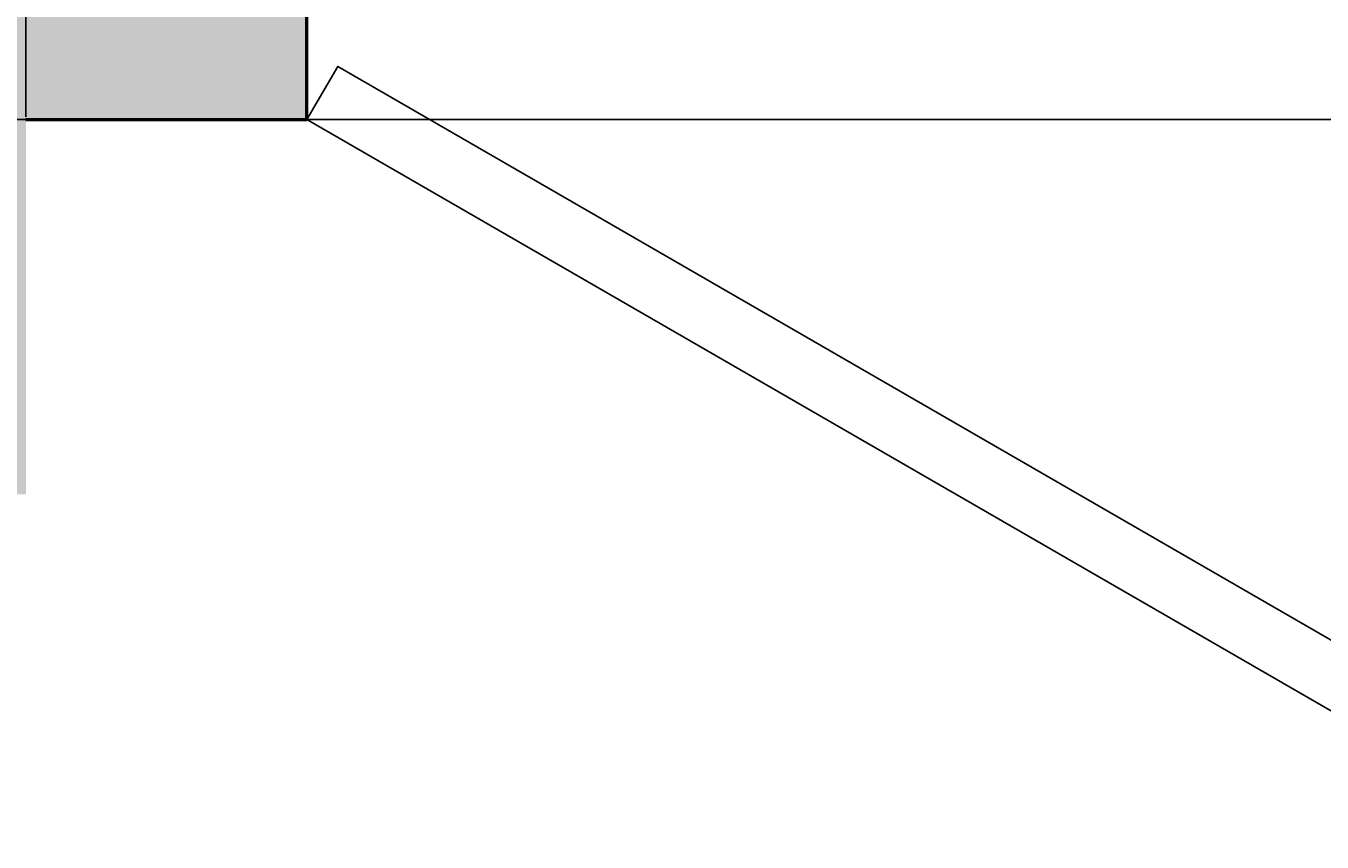
# Model space of a CAD drawing. Units: inches. Extents: x 2231 to 2461, y 2045 to 2455.
# Tile 12 of 95: x 2299 to 2326, y 2167 to 2185. Entities that reach past the tile are written whole.
import ezdxf

# ---------------------------------------------------------------- set-up
doc = ezdxf.new("R2010")
doc.units = ezdxf.units.IN
for name, color, linetype, lineweight in [('A-ANNO-DIMS', 2, 'Continuous', 18), ('A-DOOR', 3, 'Continuous', 25), ('A-WALL', 7, 'Continuous', 50)]:
    doc.layers.add(name, color=color, linetype=linetype, lineweight=lineweight)
doc.layers.add('A-WALL-PATT', color=18, linetype='Continuous', lineweight=13, true_color=0x000000)
doc.styles.get("Standard").update_dxf_attribs({"font": 'arial.ttf'})
doc.dimstyles.get("Standard").update_dxf_attribs({"dimtxt": 0.18, "dimasz": 0.18, "dimexe": 0.18, "dimexo": 0.0625, "dimgap": 0.09, "dimtad": 0, "dimtih": 1, "dimtoh": 1, "dimdec": 4, "dimzin": 0, "dimdsep": 46, "dimtxsty": 'Standard', "dimcen": 0.09, "dimadec": 0, "dimazin": 0, "dimtfac": 1, "dimtdec": 4, "dimtofl": 0, "dimtmove": 0, "dimatfit": 3, "dimfxl": 1, "dimtolj": 1, "dimtzin": 0, "dimarcsym": 0})

# ---------------------------------------------------------------- blocks, each defined once
blk = doc.blocks.new('*U4')
blk.add_line((0, 0), (0, 6))
blk.add_lwpolyline([(0, 0), (34.641, -20), (35.516, -18.484), (0.875, 1.516)], close=True)
blk = doc.blocks.new('*D49')
at = {"layer": 'A-ANNO-DIMS', "color": 0, "lineweight": -2, "transparency": 16777216}
for p, q in [((2298.794, 2182.895), (2298.794, 2454.645)), ((2304.794, 2182.895), (2304.794, 2454.645)), ((2298.974, 2454.465), (2301.644, 2454.465)), ((2304.614, 2454.465), (2301.943, 2454.465))]:
    blk.add_line(p, q, dxfattribs=at)
at = {"layer": 'A-ANNO-DIMS', "color": 0, "transparency": 16777216}
for points in [[(2298.974, 2454.495), (2298.974, 2454.435), (2298.794, 2454.465)], [(2304.614, 2454.495), (2304.614, 2454.435), (2304.794, 2454.465)]]:
    blk.add_solid(points, dxfattribs=at)
at = {"layer": 'Defpoints', "color": 0, "transparency": 16777216}
for p in [(2304.794, 2454.465), (2298.794, 2182.833), (2304.794, 2182.833)]:
    blk.add_point(p, dxfattribs=at)
at = {"layer": 'A-ANNO-DIMS', "color": 0, "transparency": 16777216, "insert": (2301.794, 2454.465), "char_height": 0.18, "attachment_point": 5}
blk.add_mtext('\\A1;6', dxfattribs=at)
blk = doc.blocks.new('*D50')
at = {"layer": 'A-ANNO-DIMS', "color": 0, "lineweight": -2, "transparency": 16777216}
for p, q in [((2304.794, 2182.895), (2304.794, 2454.645)), ((2334.794, 2182.895), (2334.794, 2454.645)), ((2304.974, 2454.465), (2319.575, 2454.465)), ((2334.614, 2454.465), (2320.012, 2454.465))]:
    blk.add_line(p, q, dxfattribs=at)
at = {"layer": 'A-ANNO-DIMS', "color": 0, "transparency": 16777216}
for points in [[(2304.974, 2454.495), (2304.974, 2454.435), (2304.794, 2454.465)], [(2334.614, 2454.495), (2334.614, 2454.435), (2334.794, 2454.465)]]:
    blk.add_solid(points, dxfattribs=at)
at = {"layer": 'Defpoints', "color": 0, "transparency": 16777216}
for p in [(2334.794, 2454.465), (2304.794, 2182.833), (2334.794, 2182.833)]:
    blk.add_point(p, dxfattribs=at)
at = {"layer": 'A-ANNO-DIMS', "color": 0, "transparency": 16777216, "insert": (2319.794, 2454.465), "char_height": 0.18, "attachment_point": 5}
blk.add_mtext('\\A1;30', dxfattribs=at)
blk = doc.blocks.new('*D51')
at = {"layer": 'A-ANNO-DIMS', "color": 0, "lineweight": -2, "transparency": 16777216}
for p, q in [((2258.794, 2306.77), (2258.794, 2044.803)), ((2330.794, 2306.77), (2330.794, 2044.803)), ((2258.974, 2044.983), (2294.576, 2044.983)), ((2330.614, 2044.983), (2295.011, 2044.983))]:
    blk.add_line(p, q, dxfattribs=at)
at = {"layer": 'A-ANNO-DIMS', "color": 0, "transparency": 16777216}
for points in [[(2258.974, 2045.013), (2258.974, 2044.953), (2258.794, 2044.983)], [(2330.614, 2045.013), (2330.614, 2044.953), (2330.794, 2044.983)]]:
    blk.add_solid(points, dxfattribs=at)
at = {"layer": 'Defpoints', "color": 0, "transparency": 16777216}
for p in [(2258.794, 2306.833), (2330.794, 2306.833), (2330.794, 2044.983)]:
    blk.add_point(p, dxfattribs=at)
at = {"layer": 'A-ANNO-DIMS', "color": 0, "transparency": 16777216, "insert": (2294.794, 2044.983), "char_height": 0.18, "attachment_point": 5}
blk.add_mtext('\\A1;72', dxfattribs=at)
blk = doc.blocks.new('*D60')
at = {"layer": 'A-ANNO-DIMS', "color": 0, "lineweight": -2, "transparency": 16777216}
for p, q in [((2432.731, 2182.833), (2230.981, 2182.833)), ((2231.161, 2182.653), (2231.161, 2166.906)), ((2231.161, 2150.795), (2231.161, 2166.542)), ((2432.731, 2150.615), (2230.981, 2150.615))]:
    blk.add_line(p, q, dxfattribs=at)
at = {"layer": 'A-ANNO-DIMS', "color": 0, "transparency": 16777216}
for points in [[(2231.131, 2182.653), (2231.191, 2182.653), (2231.161, 2182.833)], [(2231.131, 2150.795), (2231.191, 2150.795), (2231.161, 2150.615)]]:
    blk.add_solid(points, dxfattribs=at)
at = {"layer": 'Defpoints', "color": 0, "transparency": 16777216}
for p in [(2231.161, 2182.833), (2432.794, 2182.833), (2432.794, 2150.615)]:
    blk.add_point(p, dxfattribs=at)
at = {"layer": 'A-ANNO-DIMS', "color": 0, "transparency": 16777216, "insert": (2231.161, 2166.724), "char_height": 0.18, "attachment_point": 5}
blk.add_mtext('\\A1;32.22', dxfattribs=at)
blk = doc.blocks.new('*D65')
at = {"layer": 'A-ANNO-DIMS', "color": 0, "lineweight": -2, "transparency": 16777216}
for p, q in [((2285.635, 2189.285), (2285.635, 2044.803)), ((2340.667, 2189.285), (2340.667, 2044.803)), ((2285.815, 2044.983), (2312.758, 2044.983)), ((2340.487, 2044.983), (2313.545, 2044.983))]:
    blk.add_line(p, q, dxfattribs=at)
at = {"layer": 'A-ANNO-DIMS', "color": 0, "transparency": 16777216}
for points in [[(2285.815, 2045.013), (2285.815, 2044.953), (2285.635, 2044.983)], [(2340.487, 2045.013), (2340.487, 2044.953), (2340.667, 2044.983)]]:
    blk.add_solid(points, dxfattribs=at)
at = {"layer": 'Defpoints', "color": 0, "transparency": 16777216}
for p in [(2285.635, 2189.348), (2340.667, 2189.348), (2340.667, 2044.983)]:
    blk.add_point(p, dxfattribs=at)
at = {"layer": 'A-ANNO-DIMS', "color": 0, "transparency": 16777216, "insert": (2313.151, 2044.983), "char_height": 0.18, "attachment_point": 5}
blk.add_mtext('\\A1;55.03', dxfattribs=at)

msp = doc.modelspace()

# ---------------------------------------------------------------- hatches: boundary and pattern name
at = {"layer": 'A-WALL-PATT'}
h = msp.add_hatch(color=256, dxfattribs=at)
h.dxf.hatch_style = 1
h.paths.add_polyline_path([(2441.7935, 2269.1535), (2432.7935, 2269.1535), (2432.7935, 2186.8328), (2396.7935, 2186.8328), (2396.7935, 2286.8328), (2394.7935, 2286.8328), (2394.7935, 2186.8328), (2334.7935, 2186.8328), (2334.7935, 2182.8328), (2432.7935, 2182.8328), (2432.7935, 2072.8328), (2416.6639, 2072.8328), (2416.6639, 2063.8328), (2441.7935, 2063.8328)])
h.paths.add_polyline_path([(2368.6639, 2072.8328), (2367.04, 2072.8328), (2330.7942, 2072.8328), (2330.7397, 2063.8328), (2368.6639, 2063.8328)])
h.paths.add_polyline_path([(2300.7392, 2068.3328), (2300.7392, 2072.8328), (2298.7935, 2072.8328), (2294.7935, 2072.8328), (2258.7935, 2072.8328), (2258.7935, 2120.8328), (2294.7935, 2120.8328), (2298.7935, 2120.8328), (2298.7935, 2128.8328), (2294.7935, 2128.8328), (2294.7935, 2124.8328), (2258.7935, 2124.8328), (2258.7935, 2182.8328), (2294.7935, 2182.8328), (2294.7935, 2174.8328), (2298.7935, 2174.8328), (2298.7935, 2182.8328), (2304.7935, 2182.8328), (2304.7935, 2186.8328), (2258.7935, 2186.8328), (2258.7935, 2221.999), (2249.7935, 2221.999), (2249.7935, 2063.8328), (2300.7392, 2063.8328)])
h.paths.add_polyline_path([(2391.9338, 2435.8328), (2333.82, 2435.8328), (2333.82, 2426.8328), (2368.7935, 2426.8328), (2368.7935, 2374.9508), (2368.7935, 2370.8328), (2372.3935, 2370.8328), (2372.7935, 2370.8328), (2372.7935, 2426.8328), (2391.9338, 2426.8328)])
h.paths.add_polyline_path([(2441.7935, 2435.8328), (2415.9338, 2435.8328), (2415.9338, 2426.8328), (2432.7935, 2426.8328), (2432.7935, 2334.8328), (2372.7935, 2334.8328), (2372.7935, 2346.8328), (2368.7935, 2346.8328), (2368.7935, 2306.8328), (2360.7935, 2306.8328), (2360.7935, 2302.8328), (2368.7935, 2302.8328), (2372.7935, 2302.8328), (2372.7935, 2330.8328), (2432.7935, 2330.8328), (2432.7935, 2317.1535), (2441.7935, 2317.1535)])
h.paths.add_polyline_path([(2285.82, 2435.8328), (2249.7935, 2435.8328), (2249.7935, 2269.999), (2258.7935, 2269.999), (2258.7935, 2302.8328), (2318.8168, 2302.8328), (2330.7935, 2302.8328), (2330.7935, 2306.8328), (2258.7935, 2306.8328), (2258.7935, 2426.8328), (2285.82, 2426.8328)])

# ---------------------------------------------------------------- linework, layer by layer
at = {"layer": 'A-WALL'}
for p, q in [((2304.7935, 2182.8328), (2304.7935, 2186.8328)), ((2298.7935, 2182.8328), (2304.7935, 2182.8328))]:
    msp.add_line(p, q, dxfattribs=at)

# ---------------------------------------------------------------- block references
at = {"layer": 'A-DOOR', "xscale": 0.75, "yscale": 0.75, "zscale": 0.75}
msp.add_blockref('*U4', (2304.7935, 2182.8328), dxfattribs=at)

# ---------------------------------------------------------------- dimensions: what is measured, and where the dimension line sits
at = {"layer": 'A-ANNO-DIMS'}
for base, p1, p2, override, picture, middle in [((2304.7935, 2454.4653), (2298.7935, 2182.8328), (2304.7935, 2182.8328), {"dimdec": 0, "dimlfac": 1, "dimrnd": 0, "dimzin": 0, "dimdsep": 46, "dimlunit": 2}, '*D49', (2301.7935, 2454.4653)), ((2334.7935, 2454.4653), (2304.7935, 2182.8328), (2334.7935, 2182.8328), {"dimdec": 0, "dimlfac": 1, "dimrnd": 0, "dimzin": 0, "dimdsep": 46, "dimlunit": 2}, '*D50', (2319.7935, 2454.4653)), ((2330.7935, 2044.9825), (2258.7935, 2306.8328), (2330.7935, 2306.8328), {"dimdec": 0, "dimlfac": 1, "dimrnd": 0, "dimzin": 0, "dimdsep": 46, "dimlunit": 2}, '*D51', (2294.7935, 2044.9825)), ((2340.6673, 2044.9825), (2285.6353, 2189.3477), (2340.6673, 2189.3477), {"dimdec": 2, "dimlfac": 1, "dimrnd": 0, "dimzin": 0, "dimdsep": 46, "dimlunit": 2}, '*D65', (2313.1513, 2044.9825))]:
    dim = msp.add_linear_dim(base=base, p1=p1, p2=p2, dimstyle='Standard', override=override, dxfattribs=at)
    dim.commit()
    dim.dimension.update_dxf_attribs({"geometry": picture, "text_midpoint": middle})
dim = msp.add_linear_dim(base=(2231.161, 2182.8328), p1=(2432.7935, 2150.6145), p2=(2432.7935, 2182.8328), angle=90, dimstyle='Standard', override={"dimdec": 2, "dimlfac": 1, "dimrnd": 0, "dimzin": 0, "dimdsep": 46, "dimlunit": 2}, dxfattribs=at)
dim.commit()
dim.dimension.update_dxf_attribs({"geometry": '*D60', "text_midpoint": (2231.161, 2166.7237)})

doc.saveas('drawing.dxf')
